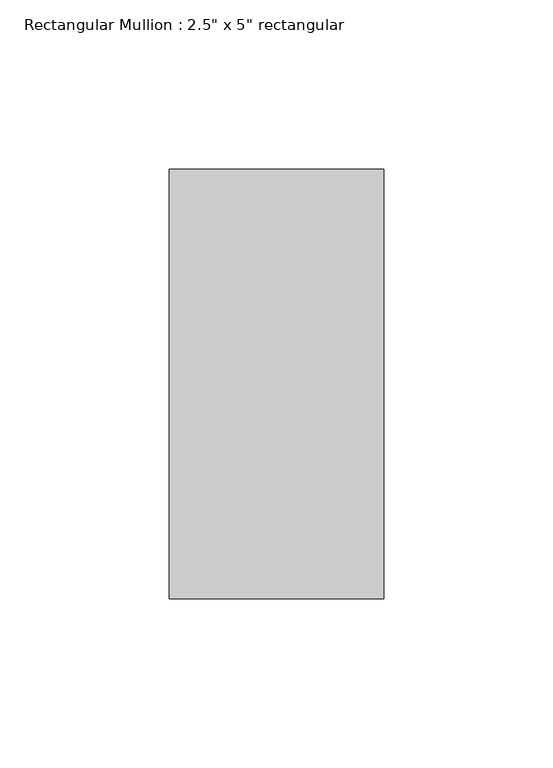
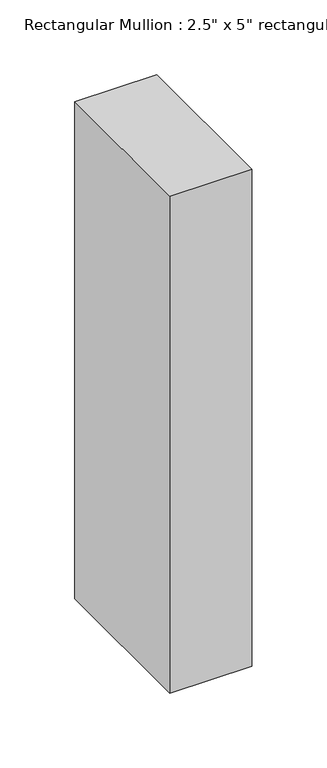
"""IFC4 building model written with IfcOpenShell, lengths in millimetres: member geometry."""

from ifc_helpers import new_model, si_unit, frame, origin, place, context, project, spatial, polyline, outline, extrude, source, transform, mapped, element, save


def member_d2428cc8(model_context):
    return source(origin(), model_context, "Body", "SweptSolid", [
        extrude(outline(polyline([(31.75, 63.5), (31.75, -63.5), (-31.75, -63.5), (-31.75, 63.5), (31.75, 63.5)])), frame((0.0, 0.0, -405.7336648), z_axis=(0.0, 0.0, 1.0), x_axis=(1.0, 0.0, 0.0)), (0.0, 0.0, 1.0), 405.7336648),
    ])


if __name__ == "__main__":
    model = new_model("IFC4")
    model_context = context("Model", 3, world=origin())
    ifc_project = project(units=[si_unit("LENGTHUNIT", "METRE", prefix="MILLI")], contexts=[model_context])
    site = spatial("IfcSite", under=ifc_project)
    building = spatial("IfcBuilding", under=site)
    placement = place(None, origin())
    member_shape = member_d2428cc8(model_context)
    element("IfcMember", 1, ObjectType="Rectangular Mullion : 2.5\" x 5\" rectangular", at=placement, inside=building, context=model_context, shape_type="MappedRepresentation", body=[
        mapped(member_shape, transform((0.0, 0.0, 0.0), x_axis=(1.0, 0.0, 0.0), y_axis=(0.0, 1.0, 0.0), z_axis=(0.0, 0.0, 1.0))),
    ])
    save(model, "model.ifc")

# Revit data of these elements
# Type "Rectangular Mullion : 2.5\" x 5\" rectangular"
#   built-in parameter 1007304 = 0.416667 (stored number, unit not read)
#   built-in parameter 1007301 = 0.104167 (stored number, unit not read)
#   built-in parameter 1007300 = 0.104167 (stored number, unit not read)
# Element 1 (IfcMember, "Rectangular Mullion : 2.5\" x 5\" rectangular")
#   Materials on its faces: "Aluminum"
# Materials
#   "Aluminum": class "Metal", colour RGB 247 247 247, transparency 0, Description = "Aluminum 6061", Cost = 0
